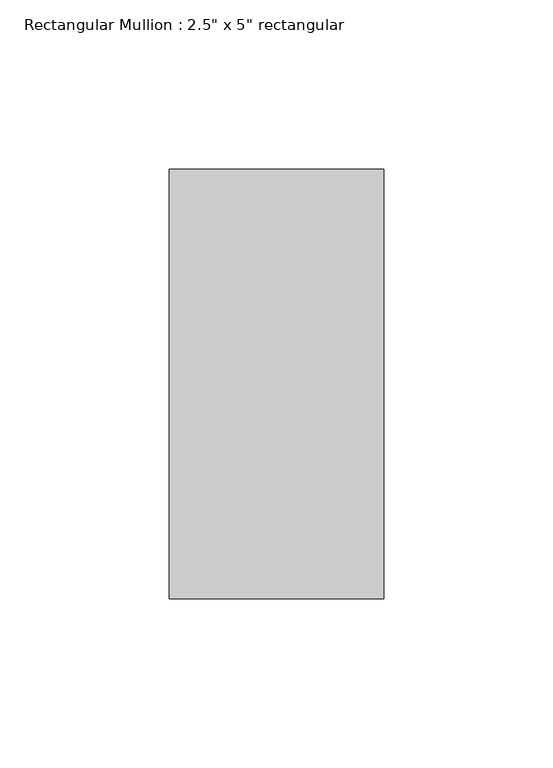
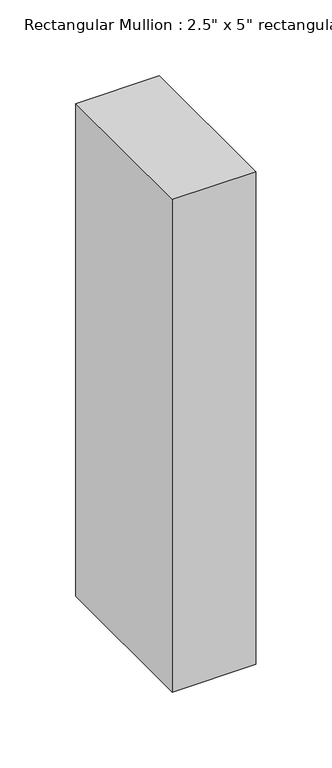
"""IFC4 building model written with IfcOpenShell, lengths in millimetres: member geometry."""

from ifc_helpers import new_model, si_unit, frame, origin, place, context, project, spatial, polyline, outline, extrude, source, transform, mapped, element, save


def member_d98df40f(model_context):
    return source(origin(), model_context, "Body", "SweptSolid", [
        extrude(outline(polyline([(0.0, 63.5), (0.0, -63.5), (-63.5, -63.5), (-63.5, 63.5), (0.0, 63.5)])), frame((0.0, 0.0, -396.24), z_axis=(0.0, 0.0, 1.0), x_axis=(1.0, 0.0, 0.0)), (0.0, 0.0, 1.0), 396.24),
    ])


if __name__ == "__main__":
    model = new_model("IFC4")
    model_context = context("Model", 3, world=origin())
    ifc_project = project(units=[si_unit("LENGTHUNIT", "METRE", prefix="MILLI")], contexts=[model_context])
    site = spatial("IfcSite", under=ifc_project)
    building = spatial("IfcBuilding", under=site)
    placement = place(None, origin())
    member_shape = member_d98df40f(model_context)
    element("IfcMember", 1, ObjectType="Rectangular Mullion : 2.5\" x 5\" rectangular", at=placement, inside=building, context=model_context, shape_type="MappedRepresentation", body=[
        mapped(member_shape, transform((0.0, 0.0, 0.0), x_axis=(1.0, 0.0, 0.0), y_axis=(0.0, 1.0, 0.0), z_axis=(0.0, 0.0, 1.0))),
    ])
    save(model, "model.ifc")

# Revit data of these elements
# Type "Rectangular Mullion : 2.5\" x 5\" rectangular"
#   built-in parameter 1007304 = 0.416667 (stored number, unit not read)
#   built-in parameter 1007301 = 0.104167 (stored number, unit not read)
#   built-in parameter 1007300 = 0.104167 (stored number, unit not read)
# Element 1 (IfcMember, "Rectangular Mullion : 2.5\" x 5\" rectangular")
#   Materials on its faces: "Aluminum"
# Materials
#   "Aluminum": class "Metal", colour RGB 247 247 247, transparency 0, Description = "Aluminum 6061", Cost = 0
